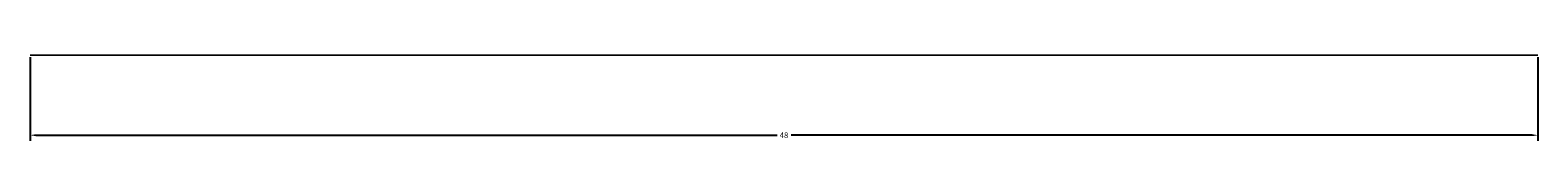
# Model space of a CAD drawing. Units: millimetres. Extents: x 3613 to 3838, y -3 to 1390.
# Tile 1 of 2: x 3790 to 3838, y -3 to 0. Entities that reach past the tile are written whole.
import ezdxf

# ---------------------------------------------------------------- set-up
doc = ezdxf.new("R2010")
doc.units = ezdxf.units.MM
doc.layers.add('M-CONS', color=7, linetype='Continuous', lineweight=18)
doc.layers.add('M-DIMS', color=2, linetype='Continuous', lineweight=18)
doc.styles.get("Standard").update_dxf_attribs({"font": 'arial.ttf'})
doc.dimstyles.get("Standard").update_dxf_attribs({"dimtxt": 0.18, "dimasz": 0.18, "dimexe": 0.18, "dimexo": 0.0625, "dimgap": 0.09, "dimtad": 0, "dimtih": 1, "dimtoh": 1, "dimdec": 4, "dimzin": 0, "dimdsep": 46, "dimtxsty": 'Standard', "dimcen": 0.09, "dimadec": 0, "dimazin": 0, "dimtfac": 1, "dimtdec": 4, "dimtofl": 0, "dimtmove": 0, "dimatfit": 3, "dimfxl": 1, "dimtolj": 1, "dimtzin": 0, "dimarcsym": 0})

# ---------------------------------------------------------------- blocks, each defined once
blk = doc.blocks.new('*D6')
at = {"layer": 'Defpoints', "color": 0, "transparency": 16777216}
for p in [(3789.536, 0), (3837.536, 0), (3837.536, -2.55)]:
    blk.add_point(p, dxfattribs=at)
at = {"layer": 'M-DIMS', "color": 0, "lineweight": -2, "transparency": 16777216}
for p, q in [((3789.536, -0.062), (3789.536, -2.73)), ((3837.536, -0.062), (3837.536, -2.73)), ((3789.716, -2.55), (3813.313, -2.55)), ((3837.356, -2.55), (3813.759, -2.55))]:
    blk.add_line(p, q, dxfattribs=at)
at = {"layer": 'M-DIMS', "color": 0, "transparency": 16777216}
for points in [[(3789.716, -2.52), (3789.716, -2.58), (3789.536, -2.55)], [(3837.356, -2.52), (3837.356, -2.58), (3837.536, -2.55)]]:
    blk.add_solid(points, dxfattribs=at)
at = {"layer": 'M-DIMS', "color": 0, "transparency": 16777216, "insert": (3813.536, -2.55), "char_height": 0.18, "attachment_point": 5}
blk.add_mtext('\\A1;48', dxfattribs=at)

msp = doc.modelspace()

# ---------------------------------------------------------------- linework, layer by layer
at = {"layer": 'M-CONS', "extrusion": (0, -1, 0)}
msp.add_lwpolyline([(3837.536, 20.268), (3837.536, 44.268, 1), (3789.536, 44.268), (3789.536, 20.268)], format="xyb", close=True, dxfattribs=at)
msp.add_circle((3813.536, 44.268), 10, dxfattribs=at)

# ---------------------------------------------------------------- dimensions: what is measured, and where the dimension line sits
at = {"layer": 'M-DIMS'}
dim = msp.add_linear_dim(base=(3837.536, -2.55), p1=(3789.536, 0), p2=(3837.536, 0), dimstyle='Standard', override={"dimdec": 0, "dimlfac": 1, "dimrnd": 0, "dimzin": 0, "dimdsep": 46, "dimlunit": 2}, dxfattribs=at)
dim.commit()
dim.dimension.update_dxf_attribs({"geometry": '*D6', "text_midpoint": (3813.536, -2.55)})

doc.saveas('drawing.dxf')
